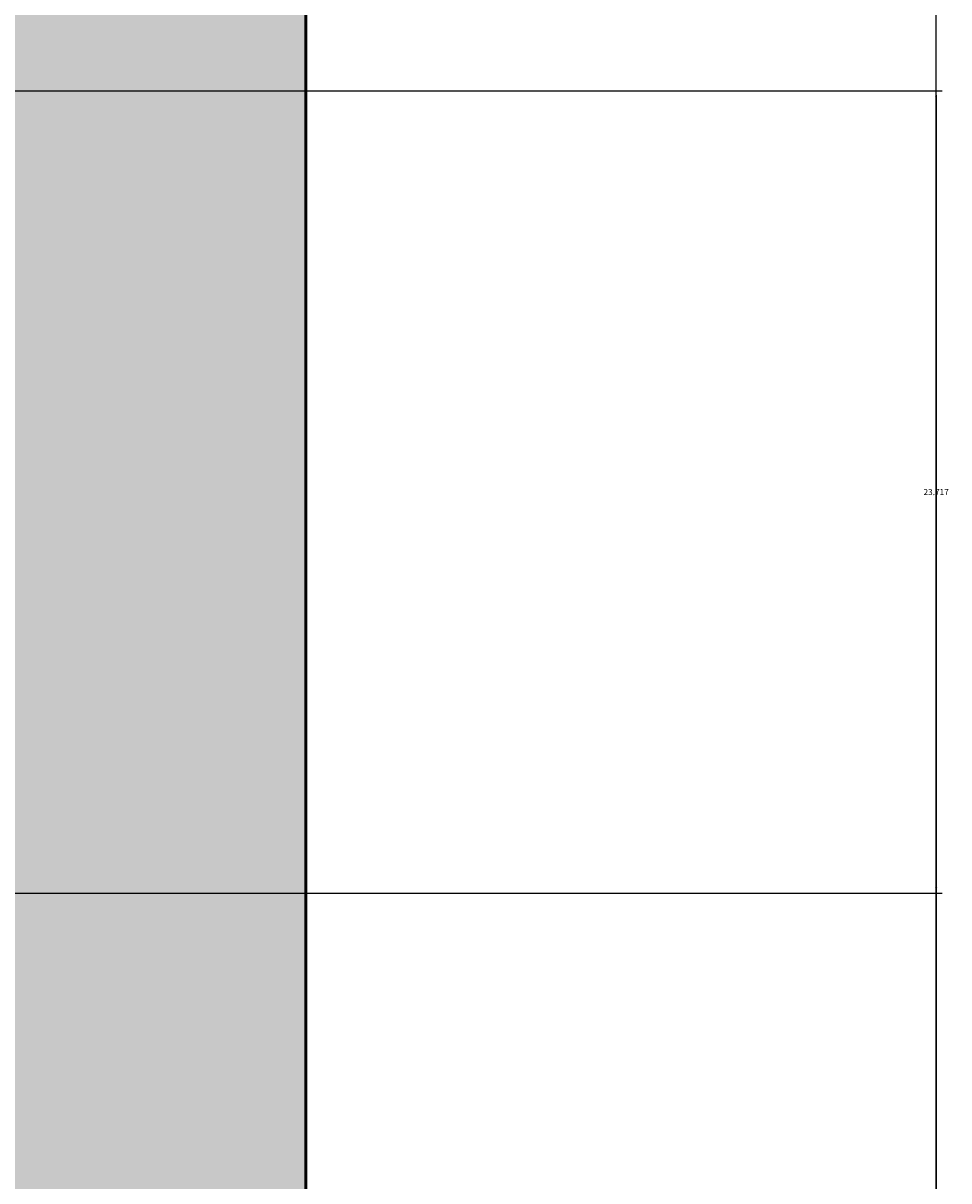
# Model space of a CAD drawing. Units: inches. Extents: x 2231 to 2461, y 2045 to 2455.
# Tile 35 of 95: x 2433 to 2461, y 2151 to 2185. Entities that reach past the tile are written whole.
import ezdxf

# ---------------------------------------------------------------- set-up
doc = ezdxf.new("R2010")
doc.units = ezdxf.units.IN
doc.layers.add('A-ANNO-DIMS', color=2, linetype='Continuous', lineweight=18)
doc.layers.add('A-WALL', color=7, linetype='Continuous', lineweight=50)
doc.layers.add('A-WALL-PATT', color=18, linetype='Continuous', lineweight=13, true_color=0x000000)
doc.styles.get("Standard").update_dxf_attribs({"font": 'arial.ttf'})
doc.dimstyles.get("Standard").update_dxf_attribs({"dimtxt": 0.18, "dimasz": 0.18, "dimexe": 0.18, "dimexo": 0.0625, "dimgap": 0.09, "dimtad": 0, "dimtih": 1, "dimtoh": 1, "dimdec": 4, "dimzin": 0, "dimdsep": 46, "dimtxsty": 'Standard', "dimcen": 0.09, "dimadec": 0, "dimazin": 0, "dimtfac": 1, "dimtdec": 4, "dimtofl": 0, "dimtmove": 0, "dimatfit": 3, "dimfxl": 1, "dimtolj": 1, "dimtzin": 0, "dimarcsym": 0})

# ---------------------------------------------------------------- blocks, each defined once
blk = doc.blocks.new('*D34')
at = {"layer": 'A-ANNO-DIMS', "color": 0, "lineweight": -2, "transparency": 16777216}
for p, q in [((2441.856, 2435.833), (2460.606, 2435.833)), ((2460.426, 2435.653), (2460.426, 2250.015)), ((2460.426, 2064.013), (2460.426, 2249.651)), ((2441.856, 2063.833), (2460.606, 2063.833))]:
    blk.add_line(p, q, dxfattribs=at)
at = {"layer": 'A-ANNO-DIMS', "color": 0, "transparency": 16777216}
for points in [[(2460.396, 2435.653), (2460.456, 2435.653), (2460.426, 2435.833)], [(2460.396, 2064.013), (2460.456, 2064.013), (2460.426, 2063.833)]]:
    blk.add_solid(points, dxfattribs=at)
at = {"layer": 'Defpoints', "color": 0, "transparency": 16777216}
for p in [(2441.794, 2435.833), (2460.426, 2435.833), (2441.794, 2063.833)]:
    blk.add_point(p, dxfattribs=at)
at = {"layer": 'A-ANNO-DIMS', "color": 0, "transparency": 16777216, "insert": (2460.426, 2249.833), "char_height": 0.18, "attachment_point": 5}
blk.add_mtext('\\A1;372', dxfattribs=at)
blk = doc.blocks.new('*D41')
at = {"layer": 'A-ANNO-DIMS', "color": 0, "lineweight": -2, "transparency": 16777216}
for p, q in [((2432.856, 2182.833), (2460.606, 2182.833)), ((2460.426, 2182.653), (2460.426, 2128.015)), ((2460.426, 2073.013), (2460.426, 2127.651)), ((2432.856, 2072.833), (2460.606, 2072.833))]:
    blk.add_line(p, q, dxfattribs=at)
at = {"layer": 'A-ANNO-DIMS', "color": 0, "transparency": 16777216}
for points in [[(2460.396, 2182.653), (2460.456, 2182.653), (2460.426, 2182.833)], [(2460.396, 2073.013), (2460.456, 2073.013), (2460.426, 2072.833)]]:
    blk.add_solid(points, dxfattribs=at)
at = {"layer": 'Defpoints', "color": 0, "transparency": 16777216}
for p in [(2432.794, 2182.833), (2460.426, 2182.833), (2432.794, 2072.833)]:
    blk.add_point(p, dxfattribs=at)
at = {"layer": 'A-ANNO-DIMS', "color": 0, "transparency": 16777216, "insert": (2460.426, 2127.833), "char_height": 0.18, "attachment_point": 5}
blk.add_mtext('\\A1;110', dxfattribs=at)
blk = doc.blocks.new('*D73')
at = {"layer": 'A-ANNO-DIMS', "color": 0, "lineweight": -2, "transparency": 16777216}
for p, q in [((2334.856, 2182.833), (2460.606, 2182.833)), ((2460.426, 2182.653), (2460.426, 2171.156)), ((2460.426, 2159.295), (2460.426, 2170.792)), ((2353.872, 2159.115), (2460.606, 2159.115))]:
    blk.add_line(p, q, dxfattribs=at)
at = {"layer": 'A-ANNO-DIMS', "color": 0, "transparency": 16777216}
for points in [[(2460.396, 2182.653), (2460.456, 2182.653), (2460.426, 2182.833)], [(2460.396, 2159.295), (2460.456, 2159.295), (2460.426, 2159.115)]]:
    blk.add_solid(points, dxfattribs=at)
at = {"layer": 'Defpoints', "color": 0, "transparency": 16777216}
for p in [(2334.794, 2182.833), (2460.426, 2182.833), (2353.809, 2159.115)]:
    blk.add_point(p, dxfattribs=at)
at = {"layer": 'A-ANNO-DIMS', "color": 0, "transparency": 16777216, "insert": (2460.426, 2170.974), "char_height": 0.18, "attachment_point": 5}
blk.add_mtext('\\A1;23.717', dxfattribs=at)

msp = doc.modelspace()

# ---------------------------------------------------------------- hatches: boundary and pattern name
at = {"layer": 'A-WALL-PATT'}
h = msp.add_hatch(color=256, dxfattribs=at)
h.dxf.hatch_style = 1
h.paths.add_polyline_path([(2441.7935, 2269.1535), (2432.7935, 2269.1535), (2432.7935, 2186.8328), (2396.7935, 2186.8328), (2396.7935, 2286.8328), (2394.7935, 2286.8328), (2394.7935, 2186.8328), (2334.7935, 2186.8328), (2334.7935, 2182.8328), (2432.7935, 2182.8328), (2432.7935, 2072.8328), (2416.6639, 2072.8328), (2416.6639, 2063.8328), (2441.7935, 2063.8328)])
h.paths.add_polyline_path([(2368.6639, 2072.8328), (2367.04, 2072.8328), (2330.7942, 2072.8328), (2330.7397, 2063.8328), (2368.6639, 2063.8328)])
h.paths.add_polyline_path([(2300.7392, 2068.3328), (2300.7392, 2072.8328), (2298.7935, 2072.8328), (2294.7935, 2072.8328), (2258.7935, 2072.8328), (2258.7935, 2120.8328), (2294.7935, 2120.8328), (2298.7935, 2120.8328), (2298.7935, 2128.8328), (2294.7935, 2128.8328), (2294.7935, 2124.8328), (2258.7935, 2124.8328), (2258.7935, 2182.8328), (2294.7935, 2182.8328), (2294.7935, 2174.8328), (2298.7935, 2174.8328), (2298.7935, 2182.8328), (2304.7935, 2182.8328), (2304.7935, 2186.8328), (2258.7935, 2186.8328), (2258.7935, 2221.999), (2249.7935, 2221.999), (2249.7935, 2063.8328), (2300.7392, 2063.8328)])
h.paths.add_polyline_path([(2391.9338, 2435.8328), (2333.82, 2435.8328), (2333.82, 2426.8328), (2368.7935, 2426.8328), (2368.7935, 2374.9508), (2368.7935, 2370.8328), (2372.3935, 2370.8328), (2372.7935, 2370.8328), (2372.7935, 2426.8328), (2391.9338, 2426.8328)])
h.paths.add_polyline_path([(2441.7935, 2435.8328), (2415.9338, 2435.8328), (2415.9338, 2426.8328), (2432.7935, 2426.8328), (2432.7935, 2334.8328), (2372.7935, 2334.8328), (2372.7935, 2346.8328), (2368.7935, 2346.8328), (2368.7935, 2306.8328), (2360.7935, 2306.8328), (2360.7935, 2302.8328), (2368.7935, 2302.8328), (2372.7935, 2302.8328), (2372.7935, 2330.8328), (2432.7935, 2330.8328), (2432.7935, 2317.1535), (2441.7935, 2317.1535)])
h.paths.add_polyline_path([(2285.82, 2435.8328), (2249.7935, 2435.8328), (2249.7935, 2269.999), (2258.7935, 2269.999), (2258.7935, 2302.8328), (2318.8168, 2302.8328), (2330.7935, 2302.8328), (2330.7935, 2306.8328), (2258.7935, 2306.8328), (2258.7935, 2426.8328), (2285.82, 2426.8328)])

# ---------------------------------------------------------------- linework, layer by layer
at = {"layer": 'A-WALL'}
msp.add_lwpolyline([(2300.7392, 2063.8328), (2249.7935, 2063.8328), (2249.7935, 2435.8328), (2441.7935, 2435.8328), (2441.7935, 2063.8328), (2330.7397, 2063.8328)], dxfattribs=at)

# ---------------------------------------------------------------- dimensions: what is measured, and where the dimension line sits
at = {"layer": 'A-ANNO-DIMS'}
for base, p1, p2, override, picture, middle in [((2460.426, 2435.8328), (2441.7935, 2063.8328), (2441.7935, 2435.8328), {"dimdec": 0, "dimlfac": 1, "dimrnd": 0, "dimzin": 0, "dimdsep": 46, "dimlunit": 2}, '*D34', (2460.426, 2249.8328)), ((2460.426, 2182.8328), (2353.8091, 2159.1154), (2334.7935, 2182.8328), {"dimdec": 3, "dimlfac": 1, "dimrnd": 0, "dimzin": 0, "dimdsep": 46, "dimlunit": 2}, '*D73', (2460.426, 2170.9741)), ((2460.426, 2182.8328), (2432.7935, 2072.8328), (2432.7935, 2182.8328), {"dimdec": 0, "dimlfac": 1, "dimrnd": 0, "dimzin": 0, "dimdsep": 46, "dimlunit": 2}, '*D41', (2460.426, 2127.8328))]:
    dim = msp.add_linear_dim(base=base, p1=p1, p2=p2, angle=90, dimstyle='Standard', override=override, dxfattribs=at)
    dim.commit()
    dim.dimension.update_dxf_attribs({"geometry": picture, "text_midpoint": middle})

doc.saveas('drawing.dxf')
